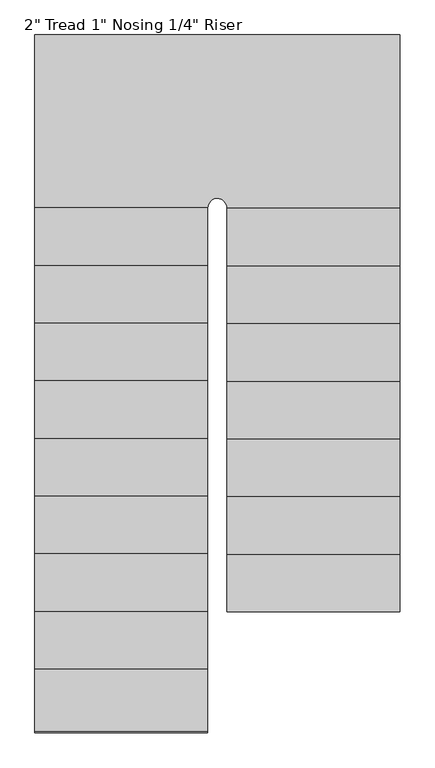
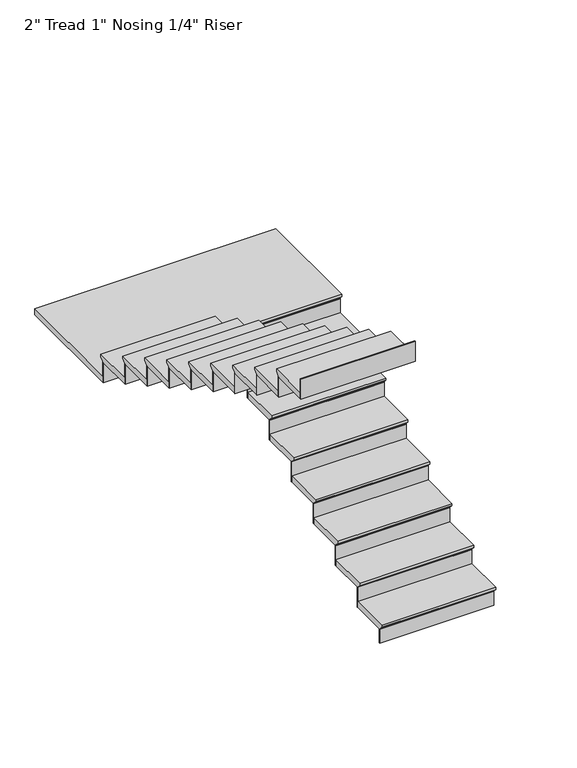
"""IFC4 building model written with IfcOpenShell, lengths in millimetres: stair flight geometry."""

from ifc_helpers import new_model, si_unit, frame, origin, place, context, project, spatial, polyline, circle_curve, ellipse_curve, faceted_brep, source, transform, mapped, element, save
from ifc_brep_helpers import plane_surface, revolved_surface, advanced_brep


def stair_flight_1848b3f0(model_context):
    return source(origin(), model_context, "Body", "SolidModel", [
        faceted_brep([(-2547.8656154, 3686.6500875, 150.2833333), (-2547.8656154, 3686.6500875, 169.3333333), (-3462.2656154, 3686.6500875, 169.3333333), (-3462.2656154, 3686.6500875, 150.2833333), (-2547.8656154, 3712.0500875, 124.8833333), (-3462.2656154, 3712.0500875, 124.8833333), (-2547.8656154, 4016.8500875, 169.3333333), (-3462.2656154, 4016.8500875, 169.3333333), (-3462.2656154, 3712.0500875, 118.5333333), (-3462.2656154, 4016.8500875, 118.5333333), (-2547.8656154, 4016.8500875, 118.5333333), (-2547.8656154, 3712.0500875, 118.5333333)], [[[0, 1, 2, 3]], [[4, 0, 3, 5]], [[2, 1, 6, 7]], [[8, 9, 10, 11]], [[2, 7, 9, 8, 5, 3]], [[8, 11, 4, 5]], [[6, 1, 0, 4, 11, 10]], [[7, 6, 10, 9]]]),
        faceted_brep([(-2547.8656154, 3712.0500875, 118.5333333), (-2547.8656154, 3712.0500875, 0.0), (-2547.8656154, 3718.4000875, 0.0), (-2547.8656154, 3718.4000875, 118.5333333), (-3462.2656154, 3712.0500875, 118.5333333), (-3462.2656154, 3718.4000875, 118.5333333), (-3462.2656154, 3718.4000875, 0.0), (-3462.2656154, 3712.0500875, 0.0)], [[[0, 1, 2, 3]], [[4, 5, 6, 7]], [[1, 0, 4, 7]], [[2, 1, 7, 6]], [[3, 2, 6, 5]], [[0, 3, 5, 4]]]),
        faceted_brep([(-2547.8656154, 4016.8500875, 287.8666667), (-2547.8656154, 4016.8500875, 118.5333333), (-2547.8656154, 4023.2000875, 118.5333333), (-2547.8656154, 4023.2000875, 287.8666667), (-3462.2656154, 4016.8500875, 287.8666667), (-3462.2656154, 4023.2000875, 287.8666667), (-3462.2656154, 4023.2000875, 118.5333333), (-3462.2656154, 4016.8500875, 118.5333333)], [[[0, 1, 2, 3]], [[4, 5, 6, 7]], [[1, 0, 4, 7]], [[2, 1, 7, 6]], [[3, 2, 6, 5]], [[0, 3, 5, 4]]]),
        faceted_brep([(-3462.2656154, 3991.4500875, 338.6666667), (-2547.8656154, 3991.4500875, 338.6666667), (-2547.8656154, 4321.6500875, 338.6666667), (-3462.2656154, 4321.6500875, 338.6666667), (-3462.2656154, 4016.8500875, 287.8666667), (-3462.2656154, 4321.6500875, 287.8666667), (-2547.8656154, 4321.6500875, 287.8666667), (-2547.8656154, 4016.8500875, 287.8666667), (-3462.2656154, 4016.8500875, 294.2166667), (-3462.2656154, 3991.4500875, 319.6166667), (-2547.8656154, 4016.8500875, 294.2166667), (-2547.8656154, 3991.4500875, 319.6166667)], [[[0, 1, 2, 3]], [[4, 5, 6, 7]], [[0, 3, 5, 4, 8, 9]], [[4, 7, 10, 8]], [[2, 1, 11, 10, 7, 6]], [[3, 2, 6, 5]], [[11, 1, 0, 9]], [[10, 11, 9, 8]]]),
        faceted_brep([(-2547.8656154, 4321.6500875, 457.2), (-2547.8656154, 4321.6500875, 287.8666667), (-2547.8656154, 4328.0000875, 287.8666667), (-2547.8656154, 4328.0000875, 457.2), (-3462.2656154, 4321.6500875, 457.2), (-3462.2656154, 4328.0000875, 457.2), (-3462.2656154, 4328.0000875, 287.8666667), (-3462.2656154, 4321.6500875, 287.8666667)], [[[0, 1, 2, 3]], [[4, 5, 6, 7]], [[1, 0, 4, 7]], [[2, 1, 7, 6]], [[3, 2, 6, 5]], [[0, 3, 5, 4]]]),
        faceted_brep([(-3462.2656154, 4296.2500875, 508.0), (-2547.8656154, 4296.2500875, 508.0), (-2547.8656154, 4626.4500875, 508.0), (-3462.2656154, 4626.4500875, 508.0), (-3462.2656154, 4321.6500875, 457.2), (-3462.2656154, 4626.4500875, 457.2), (-2547.8656154, 4626.4500875, 457.2), (-2547.8656154, 4321.6500875, 457.2), (-3462.2656154, 4321.6500875, 463.55), (-3462.2656154, 4296.2500875, 488.95), (-2547.8656154, 4321.6500875, 463.55), (-2547.8656154, 4296.2500875, 488.95)], [[[0, 1, 2, 3]], [[4, 5, 6, 7]], [[0, 3, 5, 4, 8, 9]], [[4, 7, 10, 8]], [[2, 1, 11, 10, 7, 6]], [[3, 2, 6, 5]], [[11, 1, 0, 9]], [[10, 11, 9, 8]]]),
        faceted_brep([(-2547.8656154, 4626.4500875, 626.5333333), (-2547.8656154, 4626.4500875, 457.2), (-2547.8656154, 4632.8000875, 457.2), (-2547.8656154, 4632.8000875, 626.5333333), (-3462.2656154, 4626.4500875, 626.5333333), (-3462.2656154, 4632.8000875, 626.5333333), (-3462.2656154, 4632.8000875, 457.2), (-3462.2656154, 4626.4500875, 457.2)], [[[0, 1, 2, 3]], [[4, 5, 6, 7]], [[1, 0, 4, 7]], [[2, 1, 7, 6]], [[3, 2, 6, 5]], [[0, 3, 5, 4]]]),
        faceted_brep([(-3462.2656154, 4601.0500875, 677.3333333), (-2547.8656154, 4601.0500875, 677.3333333), (-2547.8656154, 4931.2500875, 677.3333333), (-3462.2656154, 4931.2500875, 677.3333333), (-3462.2656154, 4626.4500875, 626.5333333), (-3462.2656154, 4931.2500875, 626.5333333), (-2547.8656154, 4931.2500875, 626.5333333), (-2547.8656154, 4626.4500875, 626.5333333), (-3462.2656154, 4626.4500875, 632.8833333), (-3462.2656154, 4601.0500875, 658.2833333), (-2547.8656154, 4626.4500875, 632.8833333), (-2547.8656154, 4601.0500875, 658.2833333)], [[[0, 1, 2, 3]], [[4, 5, 6, 7]], [[0, 3, 5, 4, 8, 9]], [[4, 7, 10, 8]], [[2, 1, 11, 10, 7, 6]], [[3, 2, 6, 5]], [[11, 1, 0, 9]], [[10, 11, 9, 8]]]),
        faceted_brep([(-2547.8656154, 4931.2500875, 795.8666667), (-2547.8656154, 4931.2500875, 626.5333333), (-2547.8656154, 4937.6000875, 626.5333333), (-2547.8656154, 4937.6000875, 795.8666667), (-3462.2656154, 4931.2500875, 795.8666667), (-3462.2656154, 4937.6000875, 795.8666667), (-3462.2656154, 4937.6000875, 626.5333333), (-3462.2656154, 4931.2500875, 626.5333333)], [[[0, 1, 2, 3]], [[4, 5, 6, 7]], [[1, 0, 4, 7]], [[2, 1, 7, 6]], [[3, 2, 6, 5]], [[0, 3, 5, 4]]]),
        faceted_brep([(-3462.2656154, 4905.8500875, 846.6666667), (-2547.8656154, 4905.8500875, 846.6666667), (-2547.8656154, 5236.0500875, 846.6666667), (-3462.2656154, 5236.0500875, 846.6666667), (-3462.2656154, 4931.2500875, 795.8666667), (-3462.2656154, 5236.0500875, 795.8666667), (-2547.8656154, 5236.0500875, 795.8666667), (-2547.8656154, 4931.2500875, 795.8666667), (-3462.2656154, 4931.2500875, 802.2166667), (-3462.2656154, 4905.8500875, 827.6166667), (-2547.8656154, 4931.2500875, 802.2166667), (-2547.8656154, 4905.8500875, 827.6166667)], [[[0, 1, 2, 3]], [[4, 5, 6, 7]], [[0, 3, 5, 4, 8, 9]], [[4, 7, 10, 8]], [[2, 1, 11, 10, 7, 6]], [[3, 2, 6, 5]], [[11, 1, 0, 9]], [[10, 11, 9, 8]]]),
        faceted_brep([(-2547.8656154, 5236.0500875, 965.2), (-2547.8656154, 5236.0500875, 795.8666667), (-2547.8656154, 5242.4000875, 795.8666667), (-2547.8656154, 5242.4000875, 965.2), (-3462.2656154, 5236.0500875, 965.2), (-3462.2656154, 5242.4000875, 965.2), (-3462.2656154, 5242.4000875, 795.8666667), (-3462.2656154, 5236.0500875, 795.8666667)], [[[0, 1, 2, 3]], [[4, 5, 6, 7]], [[1, 0, 4, 7]], [[2, 1, 7, 6]], [[3, 2, 6, 5]], [[0, 3, 5, 4]]]),
        faceted_brep([(-3462.2656154, 5210.6500875, 1016.0), (-2547.8656154, 5210.6500875, 1016.0), (-2547.8656154, 5540.8500875, 1016.0), (-3462.2656154, 5540.8500875, 1016.0), (-3462.2656154, 5236.0500875, 965.2), (-3462.2656154, 5540.8500875, 965.2), (-2547.8656154, 5540.8500875, 965.2), (-2547.8656154, 5236.0500875, 965.2), (-3462.2656154, 5236.0500875, 971.55), (-3462.2656154, 5210.6500875, 996.95), (-2547.8656154, 5236.0500875, 971.55), (-2547.8656154, 5210.6500875, 996.95)], [[[0, 1, 2, 3]], [[4, 5, 6, 7]], [[0, 3, 5, 4, 8, 9]], [[4, 7, 10, 8]], [[2, 1, 11, 10, 7, 6]], [[3, 2, 6, 5]], [[11, 1, 0, 9]], [[10, 11, 9, 8]]]),
        faceted_brep([(-2547.8656154, 5540.8500875, 1134.5333333), (-2547.8656154, 5540.8500875, 965.2), (-2547.8656154, 5547.2000875, 965.2), (-2547.8656154, 5547.2000875, 1134.5333333), (-3462.2656154, 5540.8500875, 1134.5333333), (-3462.2656154, 5547.2000875, 1134.5333333), (-3462.2656154, 5547.2000875, 965.2), (-3462.2656154, 5540.8500875, 965.2)], [[[0, 1, 2, 3]], [[4, 5, 6, 7]], [[1, 0, 4, 7]], [[2, 1, 7, 6]], [[3, 2, 6, 5]], [[0, 3, 5, 4]]]),
        faceted_brep([(-3462.2656154, 5515.4500875, 1185.3333333), (-2547.8656154, 5515.4500875, 1185.3333333), (-2547.8656154, 5845.6500875, 1185.3333333), (-3462.2656154, 5845.6500875, 1185.3333333), (-3462.2656154, 5540.8500875, 1134.5333333), (-3462.2656154, 5845.6500875, 1134.5333333), (-2547.8656154, 5845.6500875, 1134.5333333), (-2547.8656154, 5540.8500875, 1134.5333333), (-3462.2656154, 5540.8500875, 1140.8833333), (-3462.2656154, 5515.4500875, 1166.2833333), (-2547.8656154, 5540.8500875, 1140.8833333), (-2547.8656154, 5515.4500875, 1166.2833333)], [[[0, 1, 2, 3]], [[4, 5, 6, 7]], [[0, 3, 5, 4, 8, 9]], [[4, 7, 10, 8]], [[2, 1, 11, 10, 7, 6]], [[3, 2, 6, 5]], [[11, 1, 0, 9]], [[10, 11, 9, 8]]]),
        advanced_brep(
        [(-2547.8656154, 5845.6500875, 1303.8666667), (-2547.8656154, 5845.6500875, 1134.5333333), (-2547.8656154, 5852.0000875, 1134.5333333), (-2547.8656154, 5852.0000875, 1303.8666667), (-3469.0715249, 5845.6500875, 1303.8666667), (-3473.4098781, 5852.0000875, 1303.8666667), (-3473.4098781, 5852.0000875, 1134.5333333), (-3469.0715249, 5845.6500875, 1134.5333333)],
        [
            (0, 1),
            (1, 2),
            (2, 3),
            (3, 0),
            (4, 5, circle_curve(frame((-3513.0656154, 5820.2500875, 1303.8666667), z_axis=(0.0, 0.0, 1.0), x_axis=(1.0, 0.0, 0.0)), 50.8)),
            (5, 6),
            (6, 7, circle_curve(frame((-3513.0656154, 5820.2500875, 1134.5333333), z_axis=(0.0, 0.0, -1.0), x_axis=(1.0, 0.0, 0.0)), 50.8)),
            (7, 4),
            (0, 4),
            (7, 1),
            (6, 2),
            (5, 3),
        ],
        [
            plane_surface(frame((-2547.8656154, 5845.6500875, 1354.6666667), z_axis=(1.0, 0.0, 0.0), x_axis=(0.0, 1.0, 0.0))),
            revolved_surface(polyline([(-3462.2656153999997, 5820.2500875, 1134.5333333), (-3462.2656153999997, 5820.2500875, 1303.8666667)]), (-3513.0656154, 5820.2500875, 1303.8666667), (0.0, 0.0, -1.0)),
            plane_surface(frame((-2547.8656154, 5845.6500875, 1303.8666667), z_axis=(0.0, -1.0, 0.0), x_axis=(-1.0, 0.0, 0.0))),
            plane_surface(frame((-2547.8656154, 5845.6500875, 1134.5333333), z_axis=(0.0, 0.0, -1.0), x_axis=(-1.0, 0.0, 0.0))),
            plane_surface(frame((-2547.8656154, 5852.0000875, 1134.5333333), z_axis=(0.0, 1.0, 0.0), x_axis=(-1.0, 0.0, 0.0))),
            plane_surface(frame((-2547.8656154, 5852.0000875, 1303.8666667), z_axis=(0.0, 0.0, 1.0), x_axis=(-1.0, 0.0, 0.0))),
        ],
        [
            (0, [[1, 2, 3, 4]]),
            (1, [[5, 6, 7, 8]]),
            (2, [[-1, 9, -8, 10]]),
            (3, [[-2, -10, -7, 11]]),
            (4, [[-3, -11, -6, 12]]),
            (5, [[-4, -12, -5, -9]]),
        ],
    ),
        advanced_brep(
        [(-3563.8656154, 5794.8500875, 1354.6666667), (-3563.8656154, 5820.2500875, 1354.6666667), (-3469.0715249, 5845.6500875, 1354.6666667), (-3462.2656154, 5820.2500875, 1354.6666667), (-2547.8656154, 5820.2500875, 1354.6666667), (-2547.8656154, 6734.6500875, 1354.6666667), (-4478.2656154, 6734.6500875, 1354.6666667), (-4478.2656154, 5794.8500875, 1354.6666667), (-3563.8656154, 5820.2500875, 1303.8666667), (-3563.8656154, 5794.8500875, 1303.8666667), (-4478.2656154, 5794.8500875, 1303.8666667), (-4478.2656154, 6734.6500875, 1303.8666667), (-2547.8656154, 6734.6500875, 1303.8666667), (-2547.8656154, 5845.6500875, 1303.8666667), (-3469.0715249, 5845.6500875, 1303.8666667), (-3469.0715249, 5845.6500875, 1310.2166667), (-2547.8656154, 5845.6500875, 1310.2166667), (-2547.8656154, 5820.2500875, 1335.6166667), (-3462.2656154, 5820.2500875, 1335.6166667)],
        [
            (0, 1),
            (1, 2, circle_curve(frame((-3513.0656154, 5820.2500875, 1354.6666667), z_axis=(0.0, 0.0, -1.0), x_axis=(1.0, 0.0, 0.0)), 50.8)),
            (2, 3, circle_curve(frame((-3513.0656154, 5820.2500875, 1354.6666667), z_axis=(0.0, 0.0, -1.0), x_axis=(1.0, 0.0, 0.0)), 50.8)),
            (3, 4),
            (4, 5),
            (5, 6),
            (6, 7),
            (7, 0),
            (8, 9),
            (9, 10),
            (10, 11),
            (11, 12),
            (12, 13),
            (13, 14),
            (14, 8, circle_curve(frame((-3513.0656154, 5820.2500875, 1303.8666667), z_axis=(0.0, 0.0, 1.0), x_axis=(1.0, 0.0, 0.0)), 50.8)),
            (0, 9),
            (8, 1),
            (14, 15),
            (15, 2),
            (13, 16),
            (16, 15),
            (4, 17),
            (17, 16),
            (12, 5),
            (11, 6),
            (10, 7),
            (18, 3),
            (15, 18, ellipse_curve(frame((-3513.0656154, 5820.2500875, 1335.6166667), z_axis=(0.0, -0.7071067811865489, -0.7071067811865461), x_axis=(0.0, 0.7071067811865461, -0.7071067811865489)), 71.842049, 50.8)),
            (18, 17),
        ],
        [
            plane_surface(frame((-3563.8656154, 5820.2500875, 1354.6666667), z_axis=(0.0, 0.0, 1.0), x_axis=(0.0, 1.0, 0.0))),
            plane_surface(frame((-3563.8656154, 5820.2500875, 1303.8666667), z_axis=(0.0, 0.0, -1.0), x_axis=(0.0, -1.0, 0.0))),
            plane_surface(frame((-3563.8656154, 5794.8500875, 1354.6666667), z_axis=(1.0, 0.0, 0.0), x_axis=(0.0, 0.0, -1.0))),
            revolved_surface(polyline([(-3462.2656153999997, 5820.2500875, 1303.8666667), (-3462.2656153999997, 5820.2500875, 1354.6666667)]), (-3513.0656154, 5820.2500875, 1303.8666667), (0.0, 0.0, -1.0)),
            plane_surface(frame((-3469.0715249, 5845.6500875, 1354.6666667), z_axis=(0.0, -1.0, 0.0), x_axis=(0.0, 0.0, -1.0))),
            plane_surface(frame((-2547.8656154, 5845.6500875, 1354.6666667), z_axis=(1.0, 0.0, 0.0), x_axis=(0.0, 0.0, -1.0))),
            plane_surface(frame((-2547.8656154, 6734.6500875, 1354.6666667), z_axis=(0.0, 1.0, 0.0), x_axis=(0.0, 0.0, -1.0))),
            plane_surface(frame((-4478.2656154, 6734.6500875, 1354.6666667), z_axis=(-1.0, 0.0, 0.0), x_axis=(0.0, 0.0, -1.0))),
            plane_surface(frame((-4478.2656154, 5794.8500875, 1354.6666667), z_axis=(0.0, -1.0, 0.0), x_axis=(0.0, 0.0, -1.0))),
            revolved_surface(polyline([(-3462.2656153999997, 5820.2500875, 1284.8166666777636), (-3462.2656153999997, 5820.2500875, 1386.4166667222364)]), (-3513.0656154, 5820.2500875, 1303.8666667), (0.0, 0.0, -1.0)),
            plane_surface(frame((-2547.8656154, 5820.2500875, 1354.6666667), z_axis=(0.0, -1.0, 0.0), x_axis=(-1.0, 0.0, 0.0))),
            plane_surface(frame((-2547.8656154, 5820.2500875, 1335.6166667), z_axis=(0.0, -0.7071067811865489, -0.7071067811865461), x_axis=(-1.0, 0.0, 0.0))),
        ],
        [
            (0, [[1, 2, 3, 4, 5, 6, 7, 8]]),
            (1, [[9, 10, 11, 12, 13, 14, 15]]),
            (2, [[-1, 16, -9, 17]]),
            (3, [[-2, -17, -15, 18, 19]]),
            (4, [[-14, 20, 21, -18]]),
            (5, [[-5, 22, 23, -20, -13, 24]]),
            (6, [[-6, -24, -12, 25]]),
            (7, [[-7, -25, -11, 26]]),
            (8, [[-8, -26, -10, -16]]),
            (9, [[27, -3, -19, 28]]),
            (10, [[-22, -4, -27, 29]]),
            (11, [[-23, -29, -28, -21]]),
        ],
    ),
        faceted_brep([(-4478.2656154, 5794.8500875, 1473.2), (-4478.2656154, 5794.8500875, 1303.8666667), (-4478.2656154, 5788.5000875, 1303.8666667), (-4478.2656154, 5788.5000875, 1473.2), (-3563.8656154, 5794.8500875, 1473.2), (-3563.8656154, 5788.5000875, 1473.2), (-3563.8656154, 5788.5000875, 1303.8666667), (-3563.8656154, 5794.8500875, 1303.8666667)], [[[0, 1, 2, 3]], [[4, 5, 6, 7]], [[1, 0, 4, 7]], [[2, 1, 7, 6]], [[3, 2, 6, 5]], [[0, 3, 5, 4]]]),
        faceted_brep([(-3563.8656154, 5820.2500875, 1524.0), (-4478.2656154, 5820.2500875, 1524.0), (-4478.2656154, 5490.0500875, 1524.0), (-3563.8656154, 5490.0500875, 1524.0), (-3563.8656154, 5794.8500875, 1473.2), (-3563.8656154, 5490.0500875, 1473.2), (-4478.2656154, 5490.0500875, 1473.2), (-4478.2656154, 5794.8500875, 1473.2), (-3563.8656154, 5794.8500875, 1479.55), (-3563.8656154, 5820.2500875, 1504.95), (-4478.2656154, 5794.8500875, 1479.55), (-4478.2656154, 5820.2500875, 1504.95)], [[[0, 1, 2, 3]], [[4, 5, 6, 7]], [[0, 3, 5, 4, 8, 9]], [[4, 7, 10, 8]], [[2, 1, 11, 10, 7, 6]], [[3, 2, 6, 5]], [[11, 1, 0, 9]], [[10, 11, 9, 8]]]),
        faceted_brep([(-4478.2656154, 5490.0500875, 1642.5333333), (-4478.2656154, 5490.0500875, 1473.2), (-4478.2656154, 5483.7000875, 1473.2), (-4478.2656154, 5483.7000875, 1642.5333333), (-3563.8656154, 5490.0500875, 1642.5333333), (-3563.8656154, 5483.7000875, 1642.5333333), (-3563.8656154, 5483.7000875, 1473.2), (-3563.8656154, 5490.0500875, 1473.2)], [[[0, 1, 2, 3]], [[4, 5, 6, 7]], [[1, 0, 4, 7]], [[2, 1, 7, 6]], [[3, 2, 6, 5]], [[0, 3, 5, 4]]]),
        faceted_brep([(-3563.8656154, 5515.4500875, 1693.3333333), (-4478.2656154, 5515.4500875, 1693.3333333), (-4478.2656154, 5185.2500875, 1693.3333333), (-3563.8656154, 5185.2500875, 1693.3333333), (-3563.8656154, 5490.0500875, 1642.5333333), (-3563.8656154, 5185.2500875, 1642.5333333), (-4478.2656154, 5185.2500875, 1642.5333333), (-4478.2656154, 5490.0500875, 1642.5333333), (-3563.8656154, 5490.0500875, 1648.8833333), (-3563.8656154, 5515.4500875, 1674.2833333), (-4478.2656154, 5490.0500875, 1648.8833333), (-4478.2656154, 5515.4500875, 1674.2833333)], [[[0, 1, 2, 3]], [[4, 5, 6, 7]], [[0, 3, 5, 4, 8, 9]], [[4, 7, 10, 8]], [[2, 1, 11, 10, 7, 6]], [[3, 2, 6, 5]], [[11, 1, 0, 9]], [[10, 11, 9, 8]]]),
        faceted_brep([(-4478.2656154, 5185.2500875, 1811.8666667), (-4478.2656154, 5185.2500875, 1642.5333333), (-4478.2656154, 5178.9000875, 1642.5333333), (-4478.2656154, 5178.9000875, 1811.8666667), (-3563.8656154, 5185.2500875, 1811.8666667), (-3563.8656154, 5178.9000875, 1811.8666667), (-3563.8656154, 5178.9000875, 1642.5333333), (-3563.8656154, 5185.2500875, 1642.5333333)], [[[0, 1, 2, 3]], [[4, 5, 6, 7]], [[1, 0, 4, 7]], [[2, 1, 7, 6]], [[3, 2, 6, 5]], [[0, 3, 5, 4]]]),
        faceted_brep([(-3563.8656154, 5210.6500875, 1862.6666667), (-4478.2656154, 5210.6500875, 1862.6666667), (-4478.2656154, 4880.4500875, 1862.6666667), (-3563.8656154, 4880.4500875, 1862.6666667), (-3563.8656154, 5185.2500875, 1811.8666667), (-3563.8656154, 4880.4500875, 1811.8666667), (-4478.2656154, 4880.4500875, 1811.8666667), (-4478.2656154, 5185.2500875, 1811.8666667), (-3563.8656154, 5185.2500875, 1818.2166667), (-3563.8656154, 5210.6500875, 1843.6166667), (-4478.2656154, 5185.2500875, 1818.2166667), (-4478.2656154, 5210.6500875, 1843.6166667)], [[[0, 1, 2, 3]], [[4, 5, 6, 7]], [[0, 3, 5, 4, 8, 9]], [[4, 7, 10, 8]], [[2, 1, 11, 10, 7, 6]], [[3, 2, 6, 5]], [[11, 1, 0, 9]], [[10, 11, 9, 8]]]),
        faceted_brep([(-4478.2656154, 4880.4500875, 1981.2), (-4478.2656154, 4880.4500875, 1811.8666667), (-4478.2656154, 4874.1000875, 1811.8666667), (-4478.2656154, 4874.1000875, 1981.2), (-3563.8656154, 4880.4500875, 1981.2), (-3563.8656154, 4874.1000875, 1981.2), (-3563.8656154, 4874.1000875, 1811.8666667), (-3563.8656154, 4880.4500875, 1811.8666667)], [[[0, 1, 2, 3]], [[4, 5, 6, 7]], [[1, 0, 4, 7]], [[2, 1, 7, 6]], [[3, 2, 6, 5]], [[0, 3, 5, 4]]]),
        faceted_brep([(-3563.8656154, 4905.8500875, 2032.0), (-4478.2656154, 4905.8500875, 2032.0), (-4478.2656154, 4575.6500875, 2032.0), (-3563.8656154, 4575.6500875, 2032.0), (-3563.8656154, 4880.4500875, 1981.2), (-3563.8656154, 4575.6500875, 1981.2), (-4478.2656154, 4575.6500875, 1981.2), (-4478.2656154, 4880.4500875, 1981.2), (-3563.8656154, 4880.4500875, 1987.55), (-3563.8656154, 4905.8500875, 2012.95), (-4478.2656154, 4880.4500875, 1987.55), (-4478.2656154, 4905.8500875, 2012.95)], [[[0, 1, 2, 3]], [[4, 5, 6, 7]], [[0, 3, 5, 4, 8, 9]], [[4, 7, 10, 8]], [[2, 1, 11, 10, 7, 6]], [[3, 2, 6, 5]], [[11, 1, 0, 9]], [[10, 11, 9, 8]]]),
        faceted_brep([(-4478.2656154, 4575.6500875, 2150.5333333), (-4478.2656154, 4575.6500875, 1981.2), (-4478.2656154, 4569.3000875, 1981.2), (-4478.2656154, 4569.3000875, 2150.5333333), (-3563.8656154, 4575.6500875, 2150.5333333), (-3563.8656154, 4569.3000875, 2150.5333333), (-3563.8656154, 4569.3000875, 1981.2), (-3563.8656154, 4575.6500875, 1981.2)], [[[0, 1, 2, 3]], [[4, 5, 6, 7]], [[1, 0, 4, 7]], [[2, 1, 7, 6]], [[3, 2, 6, 5]], [[0, 3, 5, 4]]]),
        faceted_brep([(-3563.8656154, 4601.0500875, 2201.3333333), (-4478.2656154, 4601.0500875, 2201.3333333), (-4478.2656154, 4270.8500875, 2201.3333333), (-3563.8656154, 4270.8500875, 2201.3333333), (-3563.8656154, 4575.6500875, 2150.5333333), (-3563.8656154, 4270.8500875, 2150.5333333), (-4478.2656154, 4270.8500875, 2150.5333333), (-4478.2656154, 4575.6500875, 2150.5333333), (-3563.8656154, 4575.6500875, 2156.8833333), (-3563.8656154, 4601.0500875, 2182.2833333), (-4478.2656154, 4575.6500875, 2156.8833333), (-4478.2656154, 4601.0500875, 2182.2833333)], [[[0, 1, 2, 3]], [[4, 5, 6, 7]], [[0, 3, 5, 4, 8, 9]], [[4, 7, 10, 8]], [[2, 1, 11, 10, 7, 6]], [[3, 2, 6, 5]], [[11, 1, 0, 9]], [[10, 11, 9, 8]]]),
        faceted_brep([(-4478.2656154, 4270.8500875, 2319.8666667), (-4478.2656154, 4270.8500875, 2150.5333333), (-4478.2656154, 4264.5000875, 2150.5333333), (-4478.2656154, 4264.5000875, 2319.8666667), (-3563.8656154, 4270.8500875, 2319.8666667), (-3563.8656154, 4264.5000875, 2319.8666667), (-3563.8656154, 4264.5000875, 2150.5333333), (-3563.8656154, 4270.8500875, 2150.5333333)], [[[0, 1, 2, 3]], [[4, 5, 6, 7]], [[1, 0, 4, 7]], [[2, 1, 7, 6]], [[3, 2, 6, 5]], [[0, 3, 5, 4]]]),
        faceted_brep([(-3563.8656154, 4296.2500875, 2370.6666667), (-4478.2656154, 4296.2500875, 2370.6666667), (-4478.2656154, 3966.0500875, 2370.6666667), (-3563.8656154, 3966.0500875, 2370.6666667), (-3563.8656154, 4270.8500875, 2319.8666667), (-3563.8656154, 3966.0500875, 2319.8666667), (-4478.2656154, 3966.0500875, 2319.8666667), (-4478.2656154, 4270.8500875, 2319.8666667), (-3563.8656154, 4270.8500875, 2326.2166667), (-3563.8656154, 4296.2500875, 2351.6166667), (-4478.2656154, 4270.8500875, 2326.2166667), (-4478.2656154, 4296.2500875, 2351.6166667)], [[[0, 1, 2, 3]], [[4, 5, 6, 7]], [[0, 3, 5, 4, 8, 9]], [[4, 7, 10, 8]], [[2, 1, 11, 10, 7, 6]], [[3, 2, 6, 5]], [[11, 1, 0, 9]], [[10, 11, 9, 8]]]),
        faceted_brep([(-4478.2656154, 3966.0500875, 2489.2), (-4478.2656154, 3966.0500875, 2319.8666667), (-4478.2656154, 3959.7000875, 2319.8666667), (-4478.2656154, 3959.7000875, 2489.2), (-3563.8656154, 3966.0500875, 2489.2), (-3563.8656154, 3959.7000875, 2489.2), (-3563.8656154, 3959.7000875, 2319.8666667), (-3563.8656154, 3966.0500875, 2319.8666667)], [[[0, 1, 2, 3]], [[4, 5, 6, 7]], [[1, 0, 4, 7]], [[2, 1, 7, 6]], [[3, 2, 6, 5]], [[0, 3, 5, 4]]]),
        faceted_brep([(-3563.8656154, 3991.4500875, 2540.0), (-4478.2656154, 3991.4500875, 2540.0), (-4478.2656154, 3661.2500875, 2540.0), (-3563.8656154, 3661.2500875, 2540.0), (-3563.8656154, 3966.0500875, 2489.2), (-3563.8656154, 3661.2500875, 2489.2), (-4478.2656154, 3661.2500875, 2489.2), (-4478.2656154, 3966.0500875, 2489.2), (-3563.8656154, 3966.0500875, 2495.55), (-3563.8656154, 3991.4500875, 2520.95), (-4478.2656154, 3966.0500875, 2495.55), (-4478.2656154, 3991.4500875, 2520.95)], [[[0, 1, 2, 3]], [[4, 5, 6, 7]], [[0, 3, 5, 4, 8, 9]], [[4, 7, 10, 8]], [[2, 1, 11, 10, 7, 6]], [[3, 2, 6, 5]], [[11, 1, 0, 9]], [[10, 11, 9, 8]]]),
        faceted_brep([(-4478.2656154, 3661.2500875, 2658.5333333), (-4478.2656154, 3661.2500875, 2489.2), (-4478.2656154, 3654.9000875, 2489.2), (-4478.2656154, 3654.9000875, 2658.5333333), (-3563.8656154, 3661.2500875, 2658.5333333), (-3563.8656154, 3654.9000875, 2658.5333333), (-3563.8656154, 3654.9000875, 2489.2), (-3563.8656154, 3661.2500875, 2489.2)], [[[0, 1, 2, 3]], [[4, 5, 6, 7]], [[1, 0, 4, 7]], [[2, 1, 7, 6]], [[3, 2, 6, 5]], [[0, 3, 5, 4]]]),
        faceted_brep([(-3563.8656154, 3686.6500875, 2709.3333333), (-4478.2656154, 3686.6500875, 2709.3333333), (-4478.2656154, 3356.4500875, 2709.3333333), (-3563.8656154, 3356.4500875, 2709.3333333), (-3563.8656154, 3661.2500875, 2658.5333333), (-3563.8656154, 3356.4500875, 2658.5333333), (-4478.2656154, 3356.4500875, 2658.5333333), (-4478.2656154, 3661.2500875, 2658.5333333), (-3563.8656154, 3661.2500875, 2664.8833333), (-3563.8656154, 3686.6500875, 2690.2833333), (-4478.2656154, 3661.2500875, 2664.8833333), (-4478.2656154, 3686.6500875, 2690.2833333)], [[[0, 1, 2, 3]], [[4, 5, 6, 7]], [[0, 3, 5, 4, 8, 9]], [[4, 7, 10, 8]], [[2, 1, 11, 10, 7, 6]], [[3, 2, 6, 5]], [[11, 1, 0, 9]], [[10, 11, 9, 8]]]),
        faceted_brep([(-4478.2656154, 3356.4500875, 2827.8666667), (-4478.2656154, 3356.4500875, 2658.5333333), (-4478.2656154, 3350.1000875, 2658.5333333), (-4478.2656154, 3350.1000875, 2827.8666667), (-3563.8656154, 3356.4500875, 2827.8666667), (-3563.8656154, 3350.1000875, 2827.8666667), (-3563.8656154, 3350.1000875, 2658.5333333), (-3563.8656154, 3356.4500875, 2658.5333333)], [[[0, 1, 2, 3]], [[4, 5, 6, 7]], [[1, 0, 4, 7]], [[2, 1, 7, 6]], [[3, 2, 6, 5]], [[0, 3, 5, 4]]]),
        faceted_brep([(-4478.2656154, 3051.6500875, 2997.2), (-4478.2656154, 3051.6500875, 2827.8666667), (-4478.2656154, 3045.3000875, 2827.8666667), (-4478.2656154, 3045.3000875, 2997.2), (-3563.8656154, 3051.6500875, 2997.2), (-3563.8656154, 3045.3000875, 2997.2), (-3563.8656154, 3045.3000875, 2827.8666667), (-3563.8656154, 3051.6500875, 2827.8666667)], [[[0, 1, 2, 3]], [[4, 5, 6, 7]], [[1, 0, 4, 7]], [[2, 1, 7, 6]], [[3, 2, 6, 5]], [[0, 3, 5, 4]]]),
        faceted_brep([(-3563.8656154, 3381.8500875, 2878.6666667), (-4478.2656154, 3381.8500875, 2878.6666667), (-4478.2656154, 3051.6500875, 2878.6666667), (-3563.8656154, 3051.6500875, 2878.6666667), (-3563.8656154, 3356.4500875, 2827.8666667), (-3563.8656154, 3051.6500875, 2827.8666667), (-4478.2656154, 3051.6500875, 2827.8666667), (-4478.2656154, 3356.4500875, 2827.8666667), (-3563.8656154, 3356.4500875, 2834.2166667), (-3563.8656154, 3381.8500875, 2859.6166667), (-4478.2656154, 3356.4500875, 2834.2166667), (-4478.2656154, 3381.8500875, 2859.6166667)], [[[0, 1, 2, 3]], [[4, 5, 6, 7]], [[0, 3, 5, 4, 8, 9]], [[4, 7, 10, 8]], [[2, 1, 11, 10, 7, 6]], [[3, 2, 6, 5]], [[11, 1, 0, 9]], [[10, 11, 9, 8]]]),
    ])


if __name__ == "__main__":
    model = new_model("IFC4")
    model_context = context("Model", 3, world=origin())
    ifc_project = project(units=[si_unit("LENGTHUNIT", "METRE", prefix="MILLI")], contexts=[model_context])
    site = spatial("IfcSite", under=ifc_project)
    building = spatial("IfcBuilding", under=site)
    placement = place(None, origin())
    stair_flight_shape = stair_flight_1848b3f0(model_context)
    element("IfcStairFlight", 1, ObjectType="2\" Tread 1\" Nosing 1/4\" Riser", at=placement, inside=building, context=model_context, shape_type="MappedRepresentation", body=[
        mapped(stair_flight_shape, transform((0.0, 0.0, 0.0), x_axis=(1.0, 0.0, 0.0), y_axis=(0.0, 1.0, 0.0), z_axis=(0.0, 0.0, 1.0))),
    ])
    save(model, "model.ifc")
